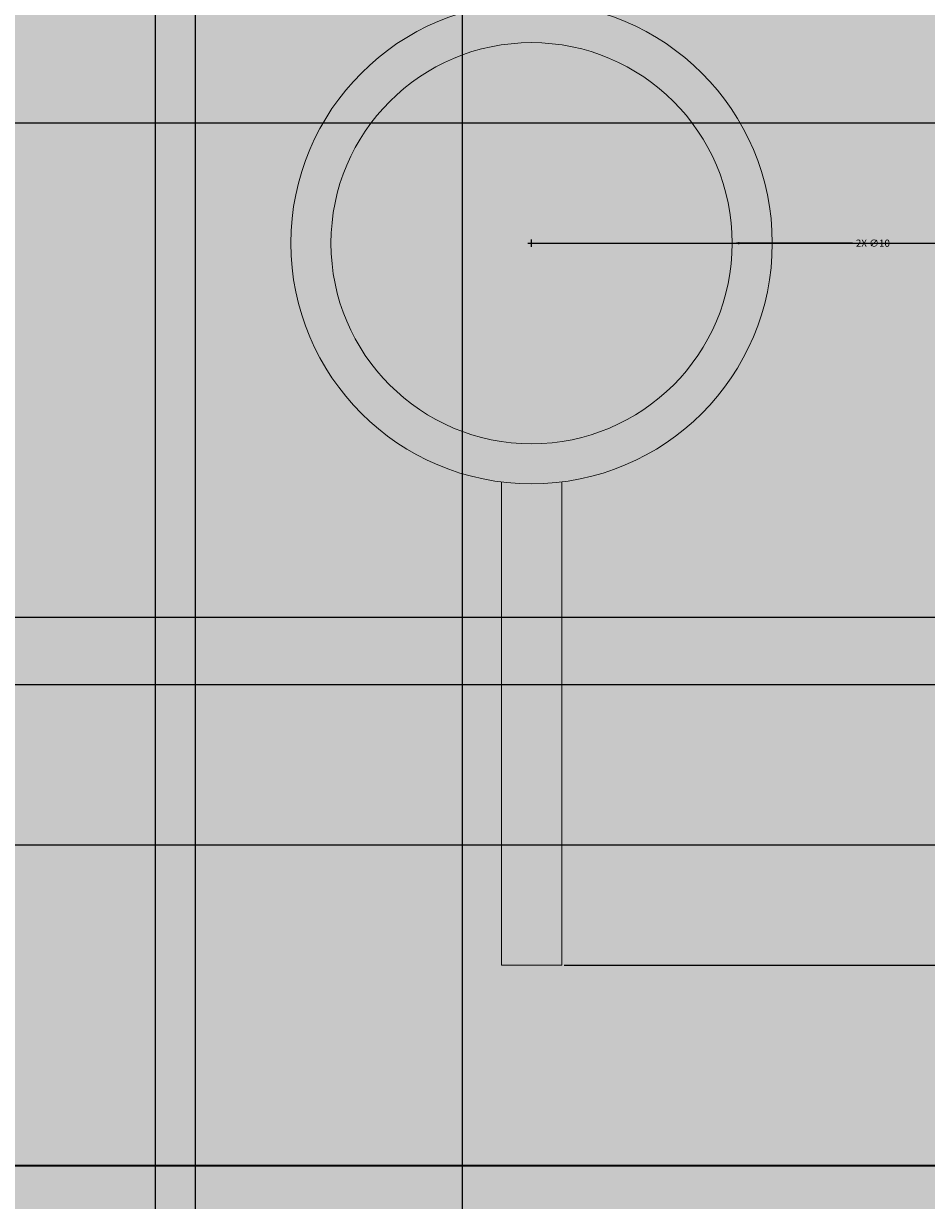
# Model space of a CAD drawing. Units: inches. Extents: x 4508 to 4723, y 847 to 1020.
# Tile 20 of 32: x 4658 to 4681, y 878 to 907. Entities that reach past the tile are written whole.
import ezdxf

# ---------------------------------------------------------------- set-up
doc = ezdxf.new("R2010")
doc.units = ezdxf.units.IN
for name, color, linetype, lineweight in [('A-ANNO-DIMS', 2, 'Continuous', 18), ('A-WALL', 7, 'Continuous', 35), ('A-WALL-DECO', 6, 'Continuous', 18), ('A-WALL-PATT', 254, 'Continuous', 13)]:
    doc.layers.add(name, color=color, linetype=linetype, lineweight=lineweight)
doc.styles.get("Standard").update_dxf_attribs({"font": 'arial.ttf'})
doc.dimstyles.get("Standard").update_dxf_attribs({"dimtxt": 0.18, "dimasz": 0.18, "dimexe": 0.18, "dimexo": 0.0625, "dimgap": 0.09, "dimtad": 0, "dimtih": 1, "dimtoh": 1, "dimdec": 4, "dimzin": 0, "dimdsep": 46, "dimtxsty": 'Standard', "dimcen": 0.09, "dimadec": 0, "dimazin": 0, "dimtfac": 1, "dimtdec": 4, "dimtofl": 0, "dimtmove": 0, "dimatfit": 3, "dimfxl": 1, "dimtolj": 1, "dimtzin": 0, "dimarcsym": 0})

# ---------------------------------------------------------------- blocks, each defined once
blk = doc.blocks.new('*D13')
at = {"layer": 'A-ANNO-DIMS', "color": 0, "lineweight": -2, "transparency": 16777216}
for p, q in [((4669.325, 973.916), (4669.325, 866.617)), ((4689.994, 874.684), (4689.994, 866.617)), ((4669.505, 866.797), (4679.264, 866.797)), ((4689.814, 866.797), (4680.054, 866.797))]:
    blk.add_line(p, q, dxfattribs=at)
at = {"layer": 'A-ANNO-DIMS', "color": 0, "lineweight": 9, "transparency": 16777216}
for points in [[(4669.505, 866.827), (4669.505, 866.767), (4669.325, 866.797)], [(4689.814, 866.827), (4689.814, 866.767), (4689.994, 866.797)]]:
    blk.add_solid(points, dxfattribs=at)
at = {"layer": 'Defpoints', "color": 0, "lineweight": 9, "transparency": 16777216}
for p in [(4669.325, 973.978), (4689.994, 874.747), (4689.994, 866.797)]:
    blk.add_point(p, dxfattribs=at)
at = {"layer": 'A-ANNO-DIMS', "color": 0, "transparency": 16777216, "insert": (4679.659, 866.797), "char_height": 0.18, "attachment_point": 5}
blk.add_mtext('\\A1;20.67', dxfattribs=at)
blk = doc.blocks.new('*D15')
at = {"layer": 'A-ANNO-DIMS', "color": 0, "lineweight": -2, "transparency": 16777216}
for p, q in [((4661.671, 918.138), (4661.671, 866.617)), ((4662.671, 918.138), (4662.671, 866.617)), ((4661.851, 866.797), (4662.047, 866.797)), ((4662.491, 866.797), (4662.294, 866.797))]:
    blk.add_line(p, q, dxfattribs=at)
at = {"layer": 'A-ANNO-DIMS', "color": 0, "lineweight": 9, "transparency": 16777216}
for points in [[(4661.851, 866.827), (4661.851, 866.767), (4661.671, 866.797)], [(4662.491, 866.827), (4662.491, 866.767), (4662.671, 866.797)]]:
    blk.add_solid(points, dxfattribs=at)
at = {"layer": 'Defpoints', "color": 0, "lineweight": 9, "transparency": 16777216}
for p in [(4661.671, 918.2), (4662.671, 918.2), (4662.671, 866.797)]:
    blk.add_point(p, dxfattribs=at)
at = {"layer": 'A-ANNO-DIMS', "color": 0, "transparency": 16777216, "insert": (4662.171, 866.797), "char_height": 0.18, "attachment_point": 5}
blk.add_mtext('\\A1;1', dxfattribs=at)
blk = doc.blocks.new('*D17')
at = {"layer": 'A-ANNO-DIMS', "color": 0, "lineweight": -2, "transparency": 16777216}
for p, q in [((4671.869, 883.747), (4702.124, 883.747)), ((4701.944, 883.567), (4701.944, 881.428)), ((4701.944, 878.927), (4701.944, 881.065)), ((4694.056, 878.747), (4702.124, 878.747))]:
    blk.add_line(p, q, dxfattribs=at)
at = {"layer": 'A-ANNO-DIMS', "color": 0, "lineweight": 9, "transparency": 16777216}
for points in [[(4701.914, 883.567), (4701.974, 883.567), (4701.944, 883.747)], [(4701.914, 878.927), (4701.974, 878.927), (4701.944, 878.747)]]:
    blk.add_solid(points, dxfattribs=at)
at = {"layer": 'Defpoints', "color": 0, "lineweight": 9, "transparency": 16777216}
for p in [(4671.806, 883.747), (4701.944, 883.747), (4693.994, 878.747)]:
    blk.add_point(p, dxfattribs=at)
at = {"layer": 'A-ANNO-DIMS', "color": 0, "transparency": 16777216, "insert": (4701.944, 881.247), "char_height": 0.18, "attachment_point": 5}
blk.add_mtext('\\A1;5', dxfattribs=at)
blk = doc.blocks.new('*D18')
at = {"layer": 'A-ANNO-DIMS', "color": 0, "lineweight": -2, "transparency": 16777216}
for p, q in [((4671.119, 901.747), (4702.124, 901.747)), ((4701.944, 901.567), (4701.944, 892.929)), ((4701.944, 883.927), (4701.944, 892.565)), ((4671.869, 883.747), (4702.124, 883.747))]:
    blk.add_line(p, q, dxfattribs=at)
at = {"layer": 'A-ANNO-DIMS', "color": 0, "lineweight": 9, "transparency": 16777216}
for points in [[(4701.914, 901.567), (4701.974, 901.567), (4701.944, 901.747)], [(4701.914, 883.927), (4701.974, 883.927), (4701.944, 883.747)]]:
    blk.add_solid(points, dxfattribs=at)
at = {"layer": 'Defpoints', "color": 0, "lineweight": 9, "transparency": 16777216}
for p in [(4671.056, 901.747), (4701.944, 901.747), (4671.806, 883.747)]:
    blk.add_point(p, dxfattribs=at)
at = {"layer": 'A-ANNO-DIMS', "color": 0, "transparency": 16777216, "insert": (4701.944, 892.747), "char_height": 0.18, "attachment_point": 5}
blk.add_mtext('\\A1;18', dxfattribs=at)
blk = doc.blocks.new('*D19')
at = {"layer": 'A-ANNO-DIMS', "color": 0, "lineweight": -2, "transparency": 16777216}
for p, q in [((4662.233, 914.641), (4702.124, 914.641)), ((4701.944, 914.461), (4701.944, 908.376)), ((4701.944, 901.927), (4701.944, 908.012)), ((4671.119, 901.747), (4702.124, 901.747))]:
    blk.add_line(p, q, dxfattribs=at)
at = {"layer": 'A-ANNO-DIMS', "color": 0, "lineweight": 9, "transparency": 16777216}
for points in [[(4701.914, 914.461), (4701.974, 914.461), (4701.944, 914.641)], [(4701.914, 901.927), (4701.974, 901.927), (4701.944, 901.747)]]:
    blk.add_solid(points, dxfattribs=at)
at = {"layer": 'Defpoints', "color": 0, "lineweight": 9, "transparency": 16777216}
for p in [(4662.171, 914.641), (4701.944, 914.641), (4671.056, 901.747)]:
    blk.add_point(p, dxfattribs=at)
at = {"layer": 'A-ANNO-DIMS', "color": 0, "transparency": 16777216, "insert": (4701.944, 908.194), "char_height": 0.18, "attachment_point": 5}
blk.add_mtext('\\A1;12.894', dxfattribs=at)
blk = doc.blocks.new('*D25')
at = {"layer": 'A-ANNO-DIMS', "color": 0, "lineweight": -2, "transparency": 16777216}
for p, q in [((4658.056, 904.747), (4702.124, 904.747)), ((4701.944, 904.567), (4701.944, 895.929)), ((4701.944, 886.927), (4701.944, 895.565)), ((4658.056, 886.747), (4702.124, 886.747))]:
    blk.add_line(p, q, dxfattribs=at)
at = {"layer": 'A-ANNO-DIMS', "color": 0, "lineweight": 9, "transparency": 16777216}
for points in [[(4701.914, 904.567), (4701.974, 904.567), (4701.944, 904.747)], [(4701.914, 886.927), (4701.974, 886.927), (4701.944, 886.747)]]:
    blk.add_solid(points, dxfattribs=at)
at = {"layer": 'Defpoints', "color": 0, "lineweight": 9, "transparency": 16777216}
for p in [(4657.994, 904.747), (4701.944, 904.747), (4657.994, 886.747)]:
    blk.add_point(p, dxfattribs=at)
at = {"layer": 'A-ANNO-DIMS', "color": 0, "transparency": 16777216, "insert": (4701.944, 895.747), "char_height": 0.18, "attachment_point": 5}
blk.add_mtext('\\A1;18', dxfattribs=at)
blk = doc.blocks.new('*D35')
at = {"layer": 'A-ANNO-DIMS', "color": 0, "lineweight": -2, "transparency": 16777216}
for p, q in [((4625.361, 892.428), (4702.124, 892.428)), ((4701.944, 892.248), (4701.944, 891.769)), ((4701.944, 890.927), (4701.944, 891.405)), ((4625.361, 890.747), (4702.124, 890.747))]:
    blk.add_line(p, q, dxfattribs=at)
at = {"layer": 'A-ANNO-DIMS', "color": 0, "lineweight": 9, "transparency": 16777216}
for points in [[(4701.914, 892.248), (4701.974, 892.248), (4701.944, 892.428)], [(4701.914, 890.927), (4701.974, 890.927), (4701.944, 890.747)]]:
    blk.add_solid(points, dxfattribs=at)
at = {"layer": 'Defpoints', "color": 0, "lineweight": 9, "transparency": 16777216}
for p in [(4625.298, 892.428), (4701.944, 892.428), (4625.298, 890.747)]:
    blk.add_point(p, dxfattribs=at)
at = {"layer": 'A-ANNO-DIMS', "color": 0, "transparency": 16777216, "insert": (4701.944, 891.587), "char_height": 0.18, "attachment_point": 5}
blk.add_mtext('\\A1;1.681', dxfattribs=at)
blk = doc.blocks.new('*D45')
at = {"layer": 'A-ANNO-DIMS', "color": 0, "lineweight": -2, "transparency": 16777216}
for p, q in [((4670.966, 901.747), (4671.146, 901.747)), ((4671.056, 901.657), (4671.056, 901.837)), ((4679.056, 901.747), (4676.236, 901.747))]:
    blk.add_line(p, q, dxfattribs=at)
at = {"layer": 'A-ANNO-DIMS', "color": 0, "lineweight": 9, "transparency": 16777216}
blk.add_solid([(4676.236, 901.777), (4676.236, 901.717), (4676.056, 901.747)], dxfattribs=at)
at = {"layer": 'Defpoints', "color": 0, "lineweight": 9, "transparency": 16777216}
for p in [(4666.056, 901.747), (4676.056, 901.747)]:
    blk.add_point(p, dxfattribs=at)
at = {"layer": 'A-ANNO-DIMS', "color": 0, "transparency": 16777216, "insert": (4679.563, 901.747), "char_height": 0.18, "attachment_point": 5}
blk.add_mtext('\\A1;2X ∅10', dxfattribs=at)

msp = doc.modelspace()

# ---------------------------------------------------------------- hatches: boundary and pattern name
at = {"layer": 'A-WALL-PATT', "transparency": 33554508}
h = msp.add_hatch(color=256, dxfattribs=at)
h.dxf.hatch_style = 1
h.paths.add_polyline_path([(4661.6706, 954.043, -0.3739004), (4658.5765, 957.6021, -1), (4665.7646, 957.6021, -0.3739004), (4662.6706, 954.043), (4662.6706, 944.4021, -0.2114781), (4670.3062, 945.0869), (4670.3062, 968.0592, -0.4632086), (4663.3246, 973.9783, -0.4632086), (4670.3062, 979.8975), (4670.3062, 994.7469), (4588.9938, 994.7469), (4588.9938, 904.7469), (4657.9938, 904.7469), (4657.9938, 886.7469), (4549.9938, 886.7469), (4549.9938, 878.7469), (4693.9938, 878.7469), (4693.9938, 994.7469), (4671.8062, 994.7469), (4671.8062, 979.4411, -0.2941682), (4675.3246, 973.9783, -0.2941682), (4671.8062, 968.5156), (4671.8062, 944.4278, -0.2741114), (4676.7298, 936.1217, -0.2741114), (4671.8062, 927.8155), (4671.8062, 907.6998, -0.3779645), (4677.0562, 901.7469, -0.3779645), (4671.8062, 895.7939), (4671.8062, 883.7469), (4670.3062, 883.7469), (4670.3062, 895.7939, -0.3779645), (4665.0562, 901.7469, -0.3779645), (4670.3062, 907.6998), (4670.3062, 927.1564, -0.2114781), (4662.6706, 927.8412), (4662.6706, 918.2003, -0.3739004), (4665.7646, 914.6412, -1), (4658.5765, 914.6412, -0.3739004), (4661.6706, 918.2003), (4661.6706, 928.4807, -0.2391825), (4657.7936, 936.1217, -0.2391825), (4661.6706, 943.7626)])
at = {"layer": 'A-WALL-PATT', "transparency": 33554556}
h = msp.add_hatch(color=256, dxfattribs=at)
h.dxf.hatch_style = 1
h.paths.add_polyline_path([(4676.0562, 901.7469, 1), (4666.0562, 901.7469, 1)])
h.paths.add_polyline_path([(4659.0765, 914.6412, 1), (4665.2646, 914.6412, 1)])
h.paths.add_polyline_path([(4675.7298, 936.1217, 1), (4658.7936, 936.1217, 1)])
h.paths.add_polyline_path([(4659.0765, 957.6021, 1), (4665.2646, 957.6021, 1)])
h.paths.add_polyline_path([(4664.3246, 973.9783, 1), (4674.3246, 973.9783, 1)])
at = {"layer": 'A-WALL-PATT', "transparency": 33554681}
h = msp.add_hatch(color=256, dxfattribs=at)
h.dxf.hatch_style = 1
h.paths.add_polyline_path([(4677.0562, 901.7469, 1), (4665.0562, 901.7469, 1)])
h.paths.add_polyline_path([(4666.0562, 901.7469, -1), (4676.0562, 901.7469, -1)], flags=16)
h = msp.add_hatch(color=256, dxfattribs=at)
h.dxf.hatch_style = 1
h.paths.add_polyline_path([(4671.8062, 895.7939, -0.0627461), (4670.3062, 895.7939), (4670.3062, 883.7469), (4671.8062, 883.7469)])
at = {"layer": 'A-WALL-PATT', "transparency": 33554556}
h = msp.add_hatch(color=256, dxfattribs=at)
h.dxf.hatch_style = 1
h.paths.add_polyline_path([(4689.9938, 878.7469), (4549.9938, 878.7469), (4549.9938, 874.7469), (4689.9938, 874.7469)])

# ---------------------------------------------------------------- linework, layer by layer
at = {"layer": 'A-WALL'}
msp.add_line((4693.9938, 878.7469), (4549.9938, 878.7469), dxfattribs=at)
at = {"layer": 'A-WALL-DECO'}
for p, q in [((4670.3062, 895.7939), (4670.3062, 883.7469)), ((4671.8062, 883.7469), (4671.8062, 895.7939)), ((4670.3062, 883.7469), (4671.8062, 883.7469))]:
    msp.add_line(p, q, dxfattribs=at)
for radius in [6, 5]:
    msp.add_circle((4671.0562, 901.7469), radius, dxfattribs=at)

# ---------------------------------------------------------------- dimensions: what is measured, and where the dimension line sits
at = {"layer": 'A-ANNO-DIMS'}
for base, p1, p2, override, picture, middle in [((4689.9938, 866.7969), (4669.3246, 973.9783), (4689.9938, 874.7469), {"dimdec": 2, "dimlfac": 1, "dimrnd": 0, "dimzin": 0, "dimdsep": 46, "dimlunit": 2}, '*D13', (4679.6592, 866.7969)), ((4662.6706, 866.7969), (4661.6706, 918.2003), (4662.6706, 918.2003), {"dimdec": 0, "dimlfac": 1, "dimrnd": 0, "dimzin": 0, "dimdsep": 46, "dimlunit": 2}, '*D15', (4662.1706, 866.7969))]:
    dim = msp.add_linear_dim(base=base, p1=p1, p2=p2, dimstyle='Standard', override=override, dxfattribs=at)
    dim.commit()
    dim.dimension.update_dxf_attribs({"geometry": picture, "text_midpoint": middle})
for base, p1, p2, override, picture, middle in [((4701.9438, 914.6412), (4671.0562, 901.7469), (4662.1706, 914.6412), {"dimdec": 3, "dimlfac": 1, "dimrnd": 0, "dimzin": 0, "dimdsep": 46, "dimlunit": 2}, '*D19', (4701.9438, 908.1941)), ((4701.9438, 904.7469), (4657.9938, 886.7469), (4657.9938, 904.7469), {"dimdec": 0, "dimlfac": 1, "dimrnd": 0, "dimzin": 0, "dimdsep": 46, "dimlunit": 2}, '*D25', (4701.9438, 895.7469)), ((4701.9438, 901.7469), (4671.8062, 883.7469), (4671.0562, 901.7469), {"dimdec": 0, "dimlfac": 1, "dimrnd": 0, "dimzin": 0, "dimdsep": 46, "dimlunit": 2}, '*D18', (4701.9438, 892.7469)), ((4701.9438, 892.4277), (4625.2983, 890.7469), (4625.2983, 892.4277), {"dimdec": 3, "dimlfac": 1, "dimrnd": 0, "dimzin": 0, "dimdsep": 46, "dimlunit": 2}, '*D35', (4701.9438, 891.5873)), ((4701.9438, 883.7469), (4693.9938, 878.7469), (4671.8062, 883.7469), {"dimdec": 0, "dimlfac": 1, "dimrnd": 0, "dimzin": 0, "dimdsep": 46, "dimlunit": 2}, '*D17', (4701.9438, 881.2469))]:
    dim = msp.add_linear_dim(base=base, p1=p1, p2=p2, angle=90, dimstyle='Standard', override=override, dxfattribs=at)
    dim.commit()
    dim.dimension.update_dxf_attribs({"geometry": picture, "text_midpoint": middle})
dim = msp.add_diameter_dim_2p(p1=(4666.0562, 901.7467), p2=(4676.0562, 901.747), text='2X <>', dimstyle='Standard', override={"dimdec": 0, "dimlfac": 1, "dimrnd": 0, "dimzin": 0, "dimdsep": 46, "dimlunit": 2}, dxfattribs=at)
dim.commit()
dim.dimension.update_dxf_attribs({"geometry": '*D45', "text_midpoint": (4679.0562, 901.7471), "dimtype": 163})

doc.saveas('drawing.dxf')
